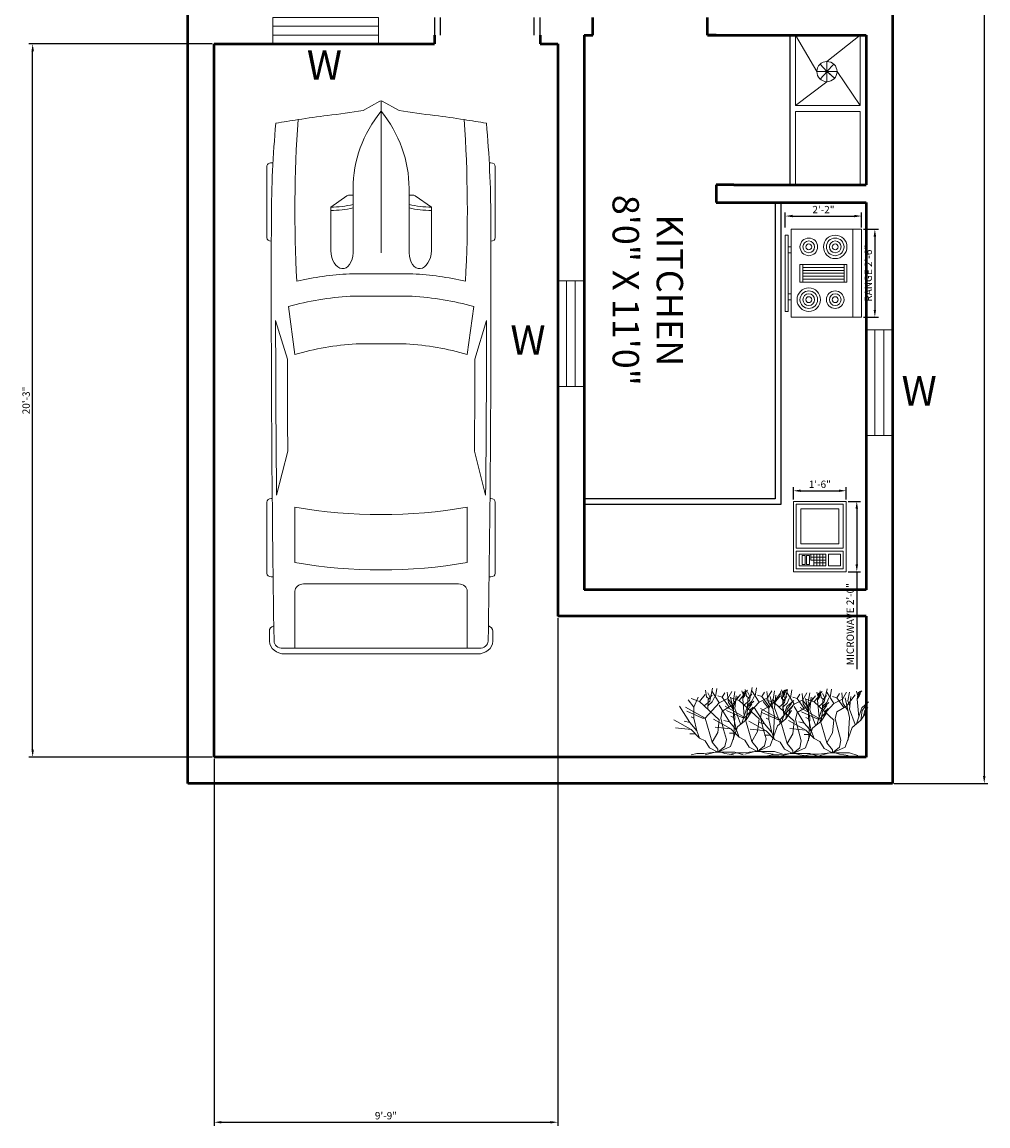
# Model space of a CAD drawing. Units: inches. Extents: x 995 to 2141, y 2161 to 2928.
# Tile 1 of 7: x 995 to 1323, y 2161 to 2537. Entities that reach past the tile are written whole.
import ezdxf

# ---------------------------------------------------------------- set-up
doc = ezdxf.new("R2010")
doc.units = ezdxf.units.IN
for name, color, linetype, lineweight in [('A-ANNO-DIMS', 2, 'Continuous', 18), ('A-ANNO-TEXT', 7, 'Continuous', 18), ('A-AREA-IDEN', 7, 'Continuous', 25), ('A-DOOR', 3, 'Continuous', 25), ('A-EQPM', 9, 'Continuous', 18), ('A-FLOR-CASE', 8, 'Continuous', 25), ('A-FLOR-FIXT', 9, 'Continuous', 18), ('A-GLAZ', 4, 'Continuous', 18), ('A-WALL', 7, 'Continuous', 50), ('C-PRKG-VEHI', 8, 'Continuous', 13), ('L-PLNT-TREE', 94, 'Continuous', 13)]:
    doc.layers.add(name, color=color, linetype=linetype, lineweight=lineweight)
doc.styles.get("Standard").update_dxf_attribs({"font": 'arial.ttf'})
doc.dimstyles.new('ISO-25', dxfattribs={"dimtxt": 2.5, "dimasz": 2.5, "dimexe": 1.25, "dimexo": 0.625, "dimtad": 1, "dimdec": 0, "dimlunit": 3, "dimtxsty": 'Standard', "dimcen": 2.5, "dimadec": 0, "dimazin": 0, "dimtfac": 1, "dimtdec": 0, "dimtmove": 0, "dimatfit": 3, "dimfxl": 1, "dimarcsym": 0})

# ---------------------------------------------------------------- blocks, each defined once
blk = doc.blocks.new('Range-Oven - 30 in top')
for p, q in [((0, -3), (30, -3)), ((12, -6), (18, -6)), ((13, -20), (13, -6)), ((14, -6), (14, -20)), ((15, -20), (15, -6)), ((16, -6), (16, -20)), ((17, -20), (17, -6)), ((18, -20), (12, -20)), ((6, -24), (6, -25)), ((8, -25), (8, -24)), ((22, -25), (22, -24)), ((24, -24), (24, -25))]:
    blk.add_line(p, q)
for points in [[(0, -24), (0, 0), (30, 0), (30, -24)], [(12, -21), (12, -5), (18, -5), (18, -21)], [(2, -26), (2, -25), (28, -25), (28, -26)]]:
    blk.add_lwpolyline(points, close=True)
for centre, radius in [((6, -9), 4), ((6, -9), 3), ((6, -9), 2), ((24, -9), 3), ((24, -9), 2), ((6, -9), 1), ((24, -9), 1), ((6, -18), 3), ((24, -18), 4), ((24, -18), 3), ((6, -18), 2), ((6, -18), 1), ((24, -18), 2), ((24, -18), 1)]:
    blk.add_circle(centre, radius)
blk = doc.blocks.new('Microwave')
for p, q in [((18, 10), (22, 10)), ((22, 9), (18, 9)), ((18, 8), (22, 8)), ((19, 7), (19, 11)), ((20, 11), (20, 7)), ((21, 7), (21, 11)), ((22, 7), (18, 7)), ((20, 6), (18, 6)), ((19, 6), (19, 7)), ((20, 7), (20, 6))]:
    blk.add_line(p, q)
for points in [[(0, 0), (0, 18), (24, 18), (24, 0)], [(1, 1), (1, 17), (16, 17), (16, 1)], [(2.5, 2.5), (2.5, 15.5), (14.5, 15.5), (14.5, 2.5)], [(17, 1), (17, 17), (23, 17), (23, 1)], [(18, 12), (18, 16), (22, 16), (22, 12)], [(18, 2), (18, 11), (22, 11), (22, 2)], [(18.5, 4.5), (18.5, 5.5), (21.5, 5.5), (21.5, 4.5)], [(18.5, 3), (18.5, 4), (21.5, 4), (21.5, 3)]]:
    blk.add_lwpolyline(points, close=True)
blk = doc.blocks.new('*U12')
for p, q in [((46.55, 38.89), (22.35, 38.89)), ((136.7, 38.89), (160.9, 38.89)), ((21.1, 37.41), (21.1, 36.83)), ((47.8, 37.39), (47.8, 37.41)), ((87.99, 31.87), (74.76, 35.92)), ((134.31, 35.6), (119.29, 31.78)), ((135.45, 37.07), (135.45, 37.41)), ((162.15, 37.41), (162.15, 36.77)), ((70.03, 31.54), (86.41, 29.35)), ((186.47, -33.5), (186.47, 33.5)), ((188.4, -32.76), (188.4, 32.76)), ((138.42, 29.35), (157.25, 29.35)), ((164.52, 26.39), (164.52, -26.39)), ((186.47, 29.35), (167.01, 29.35)), ((32.27, 11.63), (36.13, 17.17)), ((36.13, 17.17), (50.94, 17.17)), ((29.77, 9.51), (51.68, 9.51)), ((32.12, 9.51), (32.12, 11.15)), ((58.92, -10.77), (58.92, 10.77)), ((66.55, -10.53), (66.55, 10.53)), ((82.74, 8.5), (82.74, -8.5)), ((186.47, -10.53), (186.47, 10.53)), ((3.27, 6.13), (0.1, 0.41)), ((0, 0), (51.68, 0)), ((0.1, -0.41), (3.27, -6.13)), ((29.77, -9.51), (51.68, -9.51)), ((32.12, -9.51), (32.12, -11.15)), ((32.27, -11.63), (36.13, -17.17)), ((36.13, -17.17), (50.94, -17.17)), ((86.41, -29.35), (70.03, -31.54)), ((157.25, -29.35), (138.42, -29.35)), ((167.01, -29.35), (186.47, -29.35)), ((87.99, -31.87), (74.76, -35.92)), ((134.31, -35.6), (119.29, -31.78)), ((21.1, -37.41), (21.1, -36.83)), ((47.8, -37.39), (47.8, -37.41)), ((135.45, -37.07), (135.45, -37.41)), ((162.15, -37.41), (162.15, -36.77)), ((46.55, -38.89), (22.35, -38.89)), ((136.7, -38.89), (160.9, -38.89))]:
    blk.add_line(p, q)
for centre, major_axis, ratio, start_param, end_param in [((22.35, 37.41), (0, -1.48), 0.842304, 3.141593, 4.712389), ((46.55, 37.41), (0, 1.48), 0.842304, -1.570796, 0), ((136.7, 37.41), (0, -1.48), 0.842304, 3.141593, 4.712389), ((160.9, 37.41), (0, 1.48), 0.842304, -1.570796, 0), ((180.63, 35.84), (0, 2.22), 0.842304, -0.013017, 1.249894), ((64.48, -10556.36), (0, 10595.31), 0.842304, -0.013397, -0.013017), ((183.98, 32.76), (0, -5.25), 0.842304, 1.570796, 3.128196), ((266.03, -27.52), (0, 313.31), 0.842304, 1.367076, 1.39176), ((41.19, -490.86), (0, 528.23), 0.842304, 0.00281, 0.075598), ((64.48, -10555.62), (0, 10593.03), 0.842304, -0.013397, 0.002797), ((64.48, -10555.62), (0, -10591.55), 0.842304, 3.133765, 3.140441), ((183.98, 33.5), (0, -2.96), 0.842304, 1.570796, 3.128196), ((135.29, 5.39), (0, 81.77), 0.842304, 1.245306, 1.50788), ((95.79, -3666.35), (0, -3698.24), 0.842304, 3.134049, 3.144098), ((259.18, -27.52), (0, -305.3), 0.842304, 4.528606, 4.561838), ((37.47, -593.96), (0, -623.33), 0.842304, 3.096046, 3.200911), ((134.4, 5.39), (0, -89.78), 0.842304, 4.449482, 4.652344), ((149.6, 2.8), (0, -79.58), 0.842304, 4.372215, 4.640744), ((17.08, 0), (0, 147.02), 0.842304, 4.511394, 4.913384), ((35.91, 0), (0, 147.02), 0.842304, 4.511394, 4.913384), ((167.01, 26.39), (0, 2.96), 0.842304, 0, 1.570796), ((-204.49, 52.4), (0, -250.96), 0.842304, 1.385369, 1.434372), ((13.04, 17.01), (0, 27.42), 0.842304, 4.435146, 4.718221), ((14.2, 17.01), (0, 27.42), 0.842304, 4.435146, 4.718221), ((50.79, 13.34), (6.34, -0.36), 0.603834, -1.395552, 1.581315), ((32.75, 11.15), (0, 0.74), 0.842304, 0.879714, 1.570796), ((29.77, -46.66), (0, 56.17), 0.842304, 0, 0.590319), ((0.62, 0), (0, -0.74), 0.842304, 4.131459, 5.293319), ((29.77, 46.66), (0, 56.17), 0.842304, 2.551274, 3.141593), ((-204.49, -52.4), (0, 250.96), 0.842304, -1.434372, -1.385369), ((32.75, -11.15), (0, -0.74), 0.842304, 4.712389, 5.403472), ((13.04, -17.01), (0, -27.42), 0.842304, 1.564964, 1.848039), ((14.2, -17.01), (0, -27.42), 0.842304, 1.564964, 1.848039), ((134.4, -5.39), (0, -89.78), 0.842304, -1.510751, -1.307889), ((135.29, -5.39), (0, -81.77), 0.842304, -1.50788, -1.245306), ((149.6, -2.8), (0, -79.58), 0.842304, -1.499151, -1.230623), ((259.18, 27.52), (0, 305.3), 0.842304, 1.721348, 1.754579), ((266.03, 27.52), (0, 313.31), 0.842304, 1.749832, 1.774517), ((37.47, 593.96), (0, -623.33), 0.842304, -0.059319, 0.045547), ((167.01, -26.39), (0, -2.96), 0.842304, 4.712389, 6.283185), ((95.79, 3666.35), (0, -3698.24), 0.842304, -0.002505, 0.007544), ((183.98, -33.5), (0, 2.96), 0.842304, 3.15499, 4.712389), ((183.98, -32.76), (0, -5.25), 0.842304, 0.013397, 1.570796), ((41.19, 490.86), (0, -528.23), 0.842304, -0.075598, -0.00281), ((22.35, -37.41), (0, 1.48), 0.842304, 1.570796, 3.141593), ((64.48, 10555.62), (0, 10593.03), 0.842304, 3.138796, 3.15499), ((46.55, -37.41), (0, -1.48), 0.842304, 0, 1.570796), ((64.48, 10555.62), (0, -10591.55), 0.842304, 0.001152, 0.007828), ((136.7, -37.41), (0, -1.48), 0.842304, -1.570796, 0), ((160.9, -37.41), (0, 1.48), 0.842304, 3.141593, 4.712389), ((180.63, -35.84), (0, -2.22), 0.842304, -1.249894, 0.013017), ((64.48, 10556.36), (0, 10595.31), 0.842304, 3.15461, 3.15499)]:
    blk.add_ellipse(centre, major_axis=major_axis, ratio=ratio, start_param=start_param, end_param=end_param)
at = {"extrusion": (0, 0, -1)}
blk.add_ellipse((50.79, -13.34), major_axis=(6.34, 0.36), ratio=0.603834, start_param=-1.395552, end_param=1.581315, dxfattribs=at)
blk = doc.blocks.new('*U15')
for p, q in [((-11.433, 18.289), (-10.457, 22.749)), ((-9.48, 19.775), (-8.992, 22.592)), ((-14.88, 18.24), (-17.76, 19.2)), ((-16.8, 16.32), (-15.36, 19.68)), ((-14.88, 18.24), (-12.96, 20.64)), ((-12.471, 19.775), (-12.898, 22.044)), ((-11.677, 19.071), (-12.471, 19.775)), ((-11.28, 19.619), (-12.104, 21.184)), ((-12.043, 15.628), (-11.921, 18.836)), ((-11.921, 18.836), (-10.64, 20.401)), ((-10.579, 18.054), (-9.846, 19.697)), ((-8.16, 17.76), (-10.56, 21.6)), ((-7.2, 19.68), (-8.64, 20.16)), ((-8.16, 17.76), (-5.28, 19.2)), ((-7.2, 19.68), (-6.24, 21.12)), ((-4.8, 16.32), (-7.2, 19.68)), ((-5.086, 17.741), (-5.513, 21.34)), ((-5.28, 19.2), (-3.84, 21.6)), ((-2.88, 12.96), (-4.32, 19.68)), ((-3.84, 16.8), (-0.96, 20.64)), ((-3.377, 18.602), (-2.888, 21.575)), ((-2.88, 15.84), (-2.4, 20.16)), ((-0.508, 21.888), (-0.081, 20.558)), ((-0.203, 19.149), (0.102, 21.34)), ((0.346, 13.203), (-0.203, 19.149)), ((-0.142, 19.384), (0.59, 20.401)), ((-0.02, 20.01), (0.896, 21.105)), ((0.041, 20.714), (1.384, 22.044)), ((0.102, 21.34), (0.835, 21.888)), ((-18.24, 11.04), (-21.755, 16.655)), ((-12.96, 12.48), (-19.68, 16.32)), ((-16.8, 16.32), (-18.72, 18.72)), ((-16.8, 12.48), (-16.8, 16.32)), ((-8.16, 12), (-14.88, 18.24)), ((-13.325, 16.724), (-11.433, 18.289)), ((-12.96, 12.48), (-8.16, 17.76)), ((-11.982, 16.802), (-10.579, 18.054)), ((-7.2, 14.88), (-3.84, 16.8)), ((-3.377, 15.315), (-5.086, 17.819)), ((-2.766, 16.802), (-3.377, 18.602)), ((-0.96, 10.56), (-2.88, 15.84)), ((0.346, 13.203), (1.323, 16.254)), ((0.96, 12), (1.44, 15.36)), ((1.323, 16.254), (3.642, 18.289)), ((1.44, 15.36), (2.88, 17.28)), ((1.92, 13.44), (2.4, 15.36)), ((2.4, 15.36), (3.36, 16.32)), ((-17.76, 8.64), (-23.663, 11.961)), ((-18.24, 11.04), (-20.16, 11.52)), ((-13.92, 12.48), (-19.2, 14.88)), ((-16.8, 12.48), (-17.76, 12.96)), ((-15.84, 8.16), (-16.8, 12.48)), ((-12.96, 12.48), (-13.92, 12.48)), ((-10.56, 4.32), (-12.96, 12.48)), ((-8.64, 7.68), (-8.16, 12)), ((-7.68, 12.48), (-7.2, 14.88)), ((-6.72, 8.64), (-7.68, 12.48)), ((-3.36, 5.28), (-2.88, 12.96)), ((-1.92, 9.6), (0.96, 12)), ((-0.48, 10.8), (0.346, 13.203)), ((0.96, 12), (2.88, 14.88)), ((-17.76, 8.64), (-23.128, 9.222)), ((-15.84, 8.16), (-18.24, 11.04)), ((-14.88, 5.76), (-17.76, 8.64)), ((-14.88, 5.76), (-15.84, 8.16)), ((-10.56, 4.32), (-8.64, 7.68)), ((-5.76, 5.28), (-6.72, 8.64)), ((-4.32, 2.88), (-1.92, 9.6)), ((-16.32, 7.2), (-18.24, 7.2)), ((-12.96, 4.8), (-14.88, 5.76)), ((-11.52, 2.4), (-12.96, 4.8)), ((-8.64, 1.92), (-10.56, 4.32)), ((-6.24, 2.88), (-5.76, 5.28)), ((-15.84, 0.48), (-17.76, 0)), ((-13.44, 0.48), (-15.84, 0.48)), ((-9.6, 0.96), (-13.44, 0.48)), ((-9.6, 0.96), (-12.96, 0)), ((-8.64, 0.96), (-11.52, 2.4)), ((-9.6, 0.96), (-7.68, 0.96)), ((-8.64, 0.96), (-4.32, 2.88)), ((-8.64, 0.96), (-6.24, 2.88)), ((-8.64, 0.96), (-8.64, 1.92)), ((-8.64, 0.96), (-2.88, 0.96)), ((-7.68, 0.96), (-6.24, 0.48)), ((-6.24, 0.48), (-3.36, 0)), ((-2.88, 0.96), (0, 0))]:
    blk.add_line(p, q)
blk = doc.blocks.new('*D17')
at = {"layer": 'A-ANNO-DIMS', "color": 0, "lineweight": -2, "transparency": 16777216}
for p, q in [((1291.61, 2877.69), (1323.48, 2877.69)), ((1322.23, 2875.19), (1322.23, 2280.19)), ((1291.61, 2277.69), (1323.48, 2277.69))]:
    blk.add_line(p, q, dxfattribs=at)
at = {"layer": 'A-ANNO-DIMS', "color": 0, "transparency": 16777216}
for points in [[(1321.81, 2875.19), (1322.65, 2875.19), (1322.23, 2877.69)], [(1321.81, 2280.19), (1322.65, 2280.19), (1322.23, 2277.69)]]:
    blk.add_solid(points, dxfattribs=at)
at = {"layer": 'Defpoints', "color": 0, "transparency": 16777216}
for p in [(1290.98, 2877.69), (1290.98, 2277.69), (1322.23, 2277.69)]:
    blk.add_point(p, dxfattribs=at)
at = {"layer": 'A-ANNO-DIMS', "color": 0, "transparency": 16777216, "insert": (1316.5, 2577.69), "char_height": 2.5, "attachment_point": 5, "rotation": 90}
blk.add_mtext("{\\H4x;50'}", dxfattribs=at)
blk = doc.blocks.new('WIN-36IN')
for p, q in [((0, 36), (0, 0)), ((9, 36), (0, 36)), ((3, 36), (3, 0)), ((6, 0), (6, 36)), ((9, 0), (9, 36)), ((0, 0), (9, 0))]:
    blk.add_line(p, q)
blk = doc.blocks.new('*D54')
at = {"layer": 'A-ANNO-DIMS', "color": 0, "lineweight": -2, "transparency": 16777216}
for p, q in [((1281.11, 2466.52), (1286.23, 2466.52)), ((1284.98, 2464.02), (1284.98, 2439.02)), ((1281.11, 2436.52), (1286.23, 2436.52))]:
    blk.add_line(p, q, dxfattribs=at)
at = {"layer": 'A-ANNO-DIMS', "color": 0, "transparency": 16777216}
for points in [[(1284.57, 2464.02), (1285.4, 2464.02), (1284.98, 2466.52)], [(1284.57, 2439.02), (1285.4, 2439.02), (1284.98, 2436.52)]]:
    blk.add_solid(points, dxfattribs=at)
at = {"layer": 'Defpoints', "color": 0, "transparency": 16777216}
for p in [(1280.48, 2466.52), (1280.48, 2436.52), (1284.98, 2436.52)]:
    blk.add_point(p, dxfattribs=at)
at = {"layer": 'A-ANNO-DIMS', "color": 0, "transparency": 16777216, "insert": (1283.07, 2451.52), "char_height": 2.5, "attachment_point": 5, "rotation": 90}
blk.add_mtext('RANGE 2\'-6"', dxfattribs=at)
blk = doc.blocks.new('*D55')
at = {"layer": 'A-ANNO-DIMS', "color": 0, "lineweight": -2, "transparency": 16777216}
for p, q in [((1254.48, 2467.14), (1254.48, 2472.27)), ((1256.98, 2471.02), (1277.98, 2471.02)), ((1280.48, 2467.14), (1280.48, 2472.27))]:
    blk.add_line(p, q, dxfattribs=at)
at = {"layer": 'A-ANNO-DIMS', "color": 0, "transparency": 16777216}
for points in [[(1256.98, 2471.44), (1256.98, 2470.6), (1254.48, 2471.02)], [(1277.98, 2471.44), (1277.98, 2470.6), (1280.48, 2471.02)]]:
    blk.add_solid(points, dxfattribs=at)
at = {"layer": 'Defpoints', "color": 0, "transparency": 16777216}
for p in [(1280.48, 2471.02), (1254.48, 2466.52), (1280.48, 2466.52)]:
    blk.add_point(p, dxfattribs=at)
at = {"layer": 'A-ANNO-DIMS', "color": 0, "transparency": 16777216, "insert": (1267.48, 2472.9), "char_height": 2.5, "attachment_point": 5}
blk.add_mtext('2\'-2"', dxfattribs=at)
blk = doc.blocks.new('*D56')
at = {"layer": 'A-ANNO-DIMS', "color": 0, "lineweight": -2, "transparency": 16777216}
for p, q in [((1275.86, 2373.82), (1280.08, 2373.82)), ((1278.83, 2371.32), (1278.83, 2352.32)), ((1275.86, 2349.82), (1280.08, 2349.82)), ((1278.83, 2349.82), (1278.83, 2316.65))]:
    blk.add_line(p, q, dxfattribs=at)
at = {"layer": 'A-ANNO-DIMS', "color": 0, "transparency": 16777216}
for points in [[(1278.41, 2371.32), (1279.25, 2371.32), (1278.83, 2373.82)], [(1278.41, 2352.32), (1279.25, 2352.32), (1278.83, 2349.82)]]:
    blk.add_solid(points, dxfattribs=at)
at = {"layer": 'Defpoints', "color": 0, "transparency": 16777216}
for p in [(1275.23, 2373.82), (1275.23, 2349.82), (1278.83, 2349.82)]:
    blk.add_point(p, dxfattribs=at)
at = {"layer": 'A-ANNO-DIMS', "color": 0, "transparency": 16777216, "insert": (1276.91, 2331.98), "char_height": 2.5, "attachment_point": 5, "rotation": 90}
blk.add_mtext('MICROWAVE 2\'-0"', dxfattribs=at)
blk = doc.blocks.new('*D57')
at = {"layer": 'A-ANNO-DIMS', "color": 0, "lineweight": -2, "transparency": 16777216}
for p, q in [((1257.23, 2374.45), (1257.23, 2378.67)), ((1259.73, 2377.42), (1272.73, 2377.42)), ((1275.23, 2374.45), (1275.23, 2378.67))]:
    blk.add_line(p, q, dxfattribs=at)
at = {"layer": 'A-ANNO-DIMS', "color": 0, "transparency": 16777216}
for points in [[(1259.73, 2377.84), (1259.73, 2377.01), (1257.23, 2377.42)], [(1272.73, 2377.84), (1272.73, 2377.01), (1275.23, 2377.42)]]:
    blk.add_solid(points, dxfattribs=at)
at = {"layer": 'Defpoints', "color": 0, "transparency": 16777216}
for p in [(1275.23, 2377.42), (1257.23, 2373.82), (1275.23, 2373.82)]:
    blk.add_point(p, dxfattribs=at)
at = {"layer": 'A-ANNO-DIMS', "color": 0, "transparency": 16777216, "insert": (1266.23, 2379.32), "char_height": 2.5, "attachment_point": 5}
blk.add_mtext('1\'-6"', dxfattribs=at)
blk = doc.blocks.new('*D60')
at = {"layer": 'A-ANNO-DIMS', "color": 0, "lineweight": -2, "transparency": 16777216}
for p, q in [((1176.98, 2334.06), (1176.98, 2161.03)), ((1059.98, 2286.06), (1059.98, 2161.03)), ((1062.48, 2162.28), (1174.48, 2162.28))]:
    blk.add_line(p, q, dxfattribs=at)
at = {"layer": 'A-ANNO-DIMS', "color": 0, "transparency": 16777216}
for points in [[(1062.48, 2162.69), (1062.48, 2161.86), (1059.98, 2162.28)], [(1174.48, 2162.69), (1174.48, 2161.86), (1176.98, 2162.28)]]:
    blk.add_solid(points, dxfattribs=at)
at = {"layer": 'Defpoints', "color": 0, "transparency": 16777216}
for p in [(1176.98, 2334.69), (1059.98, 2286.69), (1176.98, 2162.28)]:
    blk.add_point(p, dxfattribs=at)
at = {"layer": 'A-ANNO-DIMS', "color": 0, "transparency": 16777216, "insert": (1118.48, 2164.18), "char_height": 2.5, "attachment_point": 5}
blk.add_mtext('9\'-9"', dxfattribs=at)
blk = doc.blocks.new('*D61')
at = {"layer": 'A-ANNO-DIMS', "color": 0, "lineweight": -2, "transparency": 16777216}
for p, q in [((1059.36, 2529.69), (996.93, 2529.69)), ((998.18, 2289.19), (998.18, 2527.19)), ((1059.36, 2286.69), (996.93, 2286.69))]:
    blk.add_line(p, q, dxfattribs=at)
at = {"layer": 'A-ANNO-DIMS', "color": 0, "transparency": 16777216}
for points in [[(997.77, 2527.19), (998.6, 2527.19), (998.18, 2529.69)], [(997.77, 2289.19), (998.6, 2289.19), (998.18, 2286.69)]]:
    blk.add_solid(points, dxfattribs=at)
at = {"layer": 'Defpoints', "color": 0, "transparency": 16777216}
for p in [(998.18, 2529.69), (1059.98, 2529.69), (1059.98, 2286.69)]:
    blk.add_point(p, dxfattribs=at)
at = {"layer": 'A-ANNO-DIMS', "color": 0, "transparency": 16777216, "insert": (996.28, 2408.19), "char_height": 2.5, "attachment_point": 5, "rotation": 90}
blk.add_mtext('20\'-3"', dxfattribs=at)

msp = doc.modelspace()

# ---------------------------------------------------------------- linework, layer by layer
at = {"layer": 'A-DOOR'}
for p, q in [((1134.98, 2538.69), (1134.98, 2532.69)), ((1136.98, 2538.69), (1136.98, 2532.69)), ((1168.98, 2532.69), (1168.98, 2538.69)), ((1170.98, 2532.69), (1170.98, 2538.69))]:
    msp.add_line(p, q, dxfattribs=at)
at = {"layer": 'A-FLOR-CASE'}
for p, q in [((1255.98, 2532.69), (1255.98, 2481.69)), ((1250.98, 2475.69), (1250.98, 2374.69)), ((1252.98, 2475.69), (1252.98, 2372.69)), ((1250.98, 2374.69), (1185.98, 2374.69)), ((1252.98, 2372.69), (1185.98, 2372.69))]:
    msp.add_line(p, q, dxfattribs=at)
at = {"layer": 'A-FLOR-FIXT'}
for p, q in [((1257.98, 2532.69), (1257.98, 2508.69)), ((1265.23, 2520.23), (1257.98, 2532.69)), ((1257.98, 2532.69), (1265.23, 2520.23)), ((1268.67, 2523.66), (1279.98, 2532.69)), ((1279.98, 2532.69), (1279.98, 2508.69)), ((1268.67, 2523.66), (1268.67, 2516.79)), ((1268.67, 2516.79), (1268.67, 2523.66)), ((1268.67, 2520.23), (1265.23, 2520.23)), ((1265.23, 2520.23), (1272.11, 2520.23)), ((1272.11, 2520.23), (1265.23, 2520.23)), ((1265.23, 2520.23), (1268.67, 2520.23)), ((1268.67, 2520.23), (1266.35, 2522.76)), ((1266.35, 2522.76), (1268.67, 2520.23)), ((1268.71, 2520.27), (1266.35, 2517.68)), ((1268.67, 2520.23), (1270.98, 2522.77)), ((1270.98, 2522.77), (1268.67, 2520.23)), ((1268.67, 2516.79), (1268.67, 2520.23)), ((1268.67, 2520.23), (1268.67, 2516.79)), ((1268.67, 2520.23), (1271.25, 2517.96)), ((1271.25, 2517.96), (1268.71, 2520.27)), ((1272.11, 2520.23), (1279.98, 2508.69)), ((1268.67, 2516.79), (1257.98, 2508.69)), ((1257.98, 2508.69), (1268.67, 2516.79)), ((1257.98, 2508.69), (1279.98, 2508.69)), ((1257.98, 2506.69), (1279.98, 2506.69)), ((1257.98, 2506.69), (1257.98, 2481.69)), ((1279.98, 2506.69), (1279.98, 2481.69))]:
    msp.add_line(p, q, dxfattribs=at)
msp.add_circle((1268.67, 2520.23), 3.44, dxfattribs=at)
at = {"layer": 'A-WALL'}
for p, q in [((1050.98, 2277.69), (1050.98, 2877.69)), ((1290.98, 2877.69), (1290.98, 2277.69)), ((1188.98, 2532.69), (1188.98, 2538.69)), ((1227.98, 2532.69), (1227.98, 2538.69)), ((1134.98, 2532.69), (1134.98, 2529.69)), ((1170.98, 2532.69), (1170.98, 2529.69)), ((1185.98, 2532.69), (1185.98, 2374.69)), ((1185.98, 2532.69), (1185.98, 2343.69)), ((1185.98, 2532.69), (1185.98, 2343.69)), ((1185.98, 2532.69), (1188.98, 2532.69)), ((1185.98, 2532.69), (1188.98, 2532.69)), ((1230.98, 2532.69), (1227.98, 2532.69)), ((1227.98, 2532.69), (1230.98, 2532.69)), ((1230.98, 2532.69), (1236.98, 2532.69)), ((1236.98, 2532.69), (1281.98, 2532.69)), ((1281.98, 2532.69), (1281.98, 2481.69)), ((1059.98, 2286.69), (1059.98, 2529.69)), ((1059.98, 2529.69), (1134.98, 2529.69)), ((1170.98, 2529.69), (1176.98, 2529.69)), ((1176.98, 2529.69), (1176.98, 2334.69)), ((1230.98, 2481.69), (1230.98, 2475.69)), ((1236.98, 2481.69), (1230.98, 2481.69)), ((1236.98, 2481.69), (1281.98, 2481.69)), ((1230.98, 2475.69), (1281.98, 2475.69)), ((1281.98, 2475.69), (1281.98, 2343.69)), ((1185.98, 2372.69), (1185.98, 2343.69)), ((1281.98, 2343.69), (1185.98, 2343.69)), ((1281.98, 2334.69), (1176.98, 2334.69)), ((1281.98, 2334.69), (1281.98, 2286.69)), ((1281.98, 2286.69), (1059.98, 2286.69)), ((1290.98, 2277.69), (1050.98, 2277.69))]:
    msp.add_line(p, q, dxfattribs=at)

# ---------------------------------------------------------------- block references
at = {"layer": 'A-EQPM', "rotation": 270}
for name, p in [('Range-Oven - 30 in top', (1280.48, 2466.52)), ('Microwave', (1257.23, 2373.82))]:
    msp.add_blockref(name, p, dxfattribs=at)
at = {"layer": 'A-GLAZ', "rotation": 269.9999999999986}
msp.add_blockref('WIN-36IN', (1079.93, 2538.69), dxfattribs=at)
at = {"layer": 'A-GLAZ'}
for p in [(1176.98, 2412.95), (1281.98, 2396.28)]:
    msp.add_blockref('WIN-36IN', p, dxfattribs=at)
at = {"layer": 'C-PRKG-VEHI', "rotation": 270}
msp.add_blockref('*U12', (1116.84, 2510.22), dxfattribs=at)
at = {"layer": 'L-PLNT-TREE'}
for p in [(1240.17, 2287.42), (1253.69, 2287.68), (1265.69, 2286.96), (1279.2, 2287.22)]:
    msp.add_blockref('*U15', p, dxfattribs=at)

# ---------------------------------------------------------------- texts
at = {"layer": 'A-ANNO-TEXT', "char_height": 10, "attachment_point": 1}
for insert in [(1091.54, 2527.46), (1160.86, 2433.75), (1294.08, 2416.47)]:
    msp.add_mtext_dynamic_manual_height_columns('W', width=112.484, gutter_width=12.5, heights=[0], dxfattribs=dict(at, insert=insert))
at = {"layer": 'A-AREA-IDEN', "insert": (1219.67, 2494.97), "char_height": 9, "attachment_point": 1, "rotation": 270}
msp.add_mtext_dynamic_manual_height_columns('\\pxqc;KITCHEN\\P8\'0" X 11\'0"', width=98.5067, gutter_width=12.5, heights=[0], dxfattribs=at)

# ---------------------------------------------------------------- dimensions: what is measured, and where the dimension line sits
at = {"layer": 'A-ANNO-DIMS'}
for base, p1, p2, angle, text, override, picture, middle in [((1322.23, 2277.69), (1290.98, 2877.69), (1290.98, 2277.69), 90, "{\\H4x;50'}", {"dimclrd": 0, "dimclre": 0, "dimclrt": 0}, '*D17', (1316.5, 2577.69)), ((1284.98, 2436.52), (1280.48, 2466.52), (1280.48, 2436.52), 270, 'RANGE <>', {"dimdec": 1, "dimlfac": 1, "dimrnd": 0, "dimzin": 1, "dimdsep": 46, "dimlunit": 4, "dimfrac": 2}, '*D54', (1283.07, 2451.52)), ((1278.83, 2349.82), (1275.23, 2373.82), (1275.23, 2349.82), 270, 'MICROWAVE <>', {"dimdec": 1, "dimlfac": 1, "dimrnd": 0, "dimzin": 1, "dimdsep": 46, "dimlunit": 4, "dimfrac": 2}, '*D56', (1276.91, 2331.98))]:
    dim = msp.add_linear_dim(base=base, p1=p1, p2=p2, angle=angle, text=text, dimstyle='ISO-25', override=override, dxfattribs=at)
    dim.commit()
    dim.dimension.update_dxf_attribs({"geometry": picture, "text_midpoint": middle})
dim = msp.add_linear_dim(base=(998.18, 2529.69), p1=(1059.98, 2286.69), p2=(1059.98, 2529.69), angle=90, dimstyle='ISO-25', override={"dimdec": 1, "dimlfac": 1, "dimrnd": 0, "dimzin": 1, "dimdsep": 46, "dimlunit": 4, "dimfrac": 2}, dxfattribs=at)
dim.commit()
dim.dimension.update_dxf_attribs({"geometry": '*D61', "text_midpoint": (996.28, 2408.19)})
for base, p1, p2, picture, middle in [((1280.48, 2471.02), (1254.48, 2466.52), (1280.48, 2466.52), '*D55', (1267.48, 2472.9)), ((1275.23, 2377.42), (1257.23, 2373.82), (1275.23, 2373.82), '*D57', (1266.23, 2379.32)), ((1176.98, 2162.28), (1059.98, 2286.69), (1176.98, 2334.69), '*D60', (1118.48, 2164.18))]:
    dim = msp.add_linear_dim(base=base, p1=p1, p2=p2, dimstyle='ISO-25', override={"dimdec": 1, "dimlfac": 1, "dimrnd": 0, "dimzin": 1, "dimdsep": 46, "dimlunit": 4, "dimfrac": 2}, dxfattribs=at)
    dim.commit()
    dim.dimension.update_dxf_attribs({"geometry": picture, "text_midpoint": middle})

doc.saveas('drawing.dxf')
